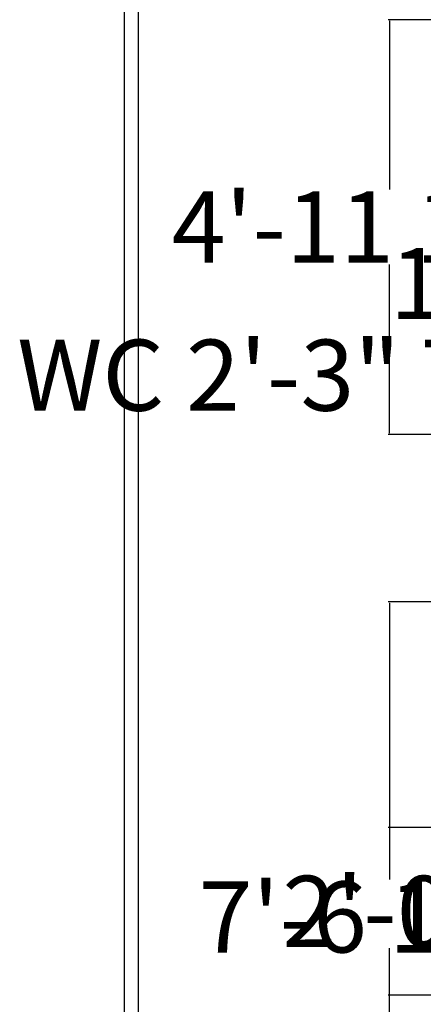
# Model space of a CAD drawing. Units: inches. Extents: x 1812 to 2791, y 2306 to 2959.
# Tile 3 of 8: x 1812 to 1870, y 2715 to 2856. Entities that reach past the tile are written whole.
import ezdxf

# ---------------------------------------------------------------- set-up
doc = ezdxf.new("R2010")
doc.units = ezdxf.units.IN
doc.layers.get('Defpoints').update_dxf_attribs({"lineweight": 50})
doc.layers.add('A-ANNO-DIMS', color=2, linetype='Continuous', lineweight=18)
doc.layers.add('A-ANNO-TTLB', color=7, linetype='Continuous', lineweight=25)
doc.styles.get("Standard").update_dxf_attribs({"font": 'arial.ttf'})
doc.dimstyles.get("Standard").update_dxf_attribs({"dimtxt": 10.18, "dimasz": 0.18, "dimexe": 0.18, "dimexo": 0.0625, "dimgap": 0.09, "dimtad": 0, "dimtih": 1, "dimtoh": 1, "dimdec": 0, "dimzin": 0, "dimdsep": 46, "dimlunit": 3, "dimtxsty": 'Standard', "dimcen": 0.09, "dimadec": 0, "dimazin": 0, "dimtfac": 1, "dimtdec": 0, "dimtofl": 0, "dimtmove": 0, "dimatfit": 3, "dimfxl": 1, "dimtolj": 1, "dimtzin": 0, "dimarcsym": 0})

# ---------------------------------------------------------------- blocks, each defined once
blk = doc.blocks.new('SHEET-FRAME-RESIDENCE')
blk.add_lwpolyline([(0.000131823559741, 632.8005012919775), (378.7609620870107, 632.8005012919775), (378.7609620870107, 0.0003856501880364), (0.000131823559741, 0.0003856501880364)], close=True)
blk.add_lwpolyline([(2.00013182355974, 71.32450104412055), (2.00013182355974, 630.8005012919775), (376.7609620870107, 630.8005012919775), (376.7609620870107, 71.32450104412055)])
blk = doc.blocks.new('*D56')
at = {"layer": 'A-ANNO-DIMS', "color": 0, "lineweight": -2, "transparency": 16777216}
for p, q in [((1900.14391049299, 2809.435242697527), (1900.14391049299, 2805.242430197514)), ((1927.312660493082, 2809.435242697527), (1927.312660493082, 2805.242430197514)), ((1900.14391049299, 2805.422430197514), (1899.96391049299, 2805.422430197514)), ((1927.132660493082, 2805.422430197514), (1900.323910492991, 2805.422430197514))]:
    blk.add_line(p, q, dxfattribs=at)
at = {"layer": 'A-ANNO-DIMS', "color": 0, "transparency": 16777216}
for points in [[(1900.323910492991, 2805.452430197514), (1900.323910492991, 2805.392430197514), (1900.14391049299, 2805.422430197514)], [(1927.132660493082, 2805.452430197514), (1927.132660493082, 2805.392430197514), (1927.312660493082, 2805.422430197514)]]:
    blk.add_solid(points, dxfattribs=at)
at = {"layer": 'Defpoints', "color": 0, "transparency": 16777216}
for p in [(1900.14391049299, 2809.497742697527), (1927.312660493082, 2809.497742697527), (1900.14391049299, 2805.422430197514)]:
    blk.add_point(p, dxfattribs=at)
at = {"layer": 'A-ANNO-DIMS', "color": 0, "transparency": 16777216, "insert": (1854.817341598038, 2805.422430197514), "char_height": 10.18, "attachment_point": 5}
blk.add_mtext('\\A1;WC 2\'-3" TYP.', dxfattribs=at)
blk = doc.blocks.new('*D57')
at = {"layer": 'A-ANNO-DIMS', "color": 0, "lineweight": -2, "transparency": 16777216}
for p, q in [((1900.081410492991, 2827.610242697545), (1895.888597992978, 2827.610242697545)), ((1896.068597992978, 2827.430242697545), (1896.068597992978, 2823.841625712543)), ((1896.068597992978, 2809.677742697528), (1896.068597992978, 2813.266359682529)), ((1900.081410492991, 2809.497742697528), (1895.888597992978, 2809.497742697528))]:
    blk.add_line(p, q, dxfattribs=at)
at = {"layer": 'A-ANNO-DIMS', "color": 0, "transparency": 16777216}
for points in [[(1896.038597992978, 2827.430242697545), (1896.098597992978, 2827.430242697545), (1896.068597992978, 2827.610242697545)], [(1896.038597992978, 2809.677742697528), (1896.098597992978, 2809.677742697528), (1896.068597992978, 2809.497742697528)]]:
    blk.add_solid(points, dxfattribs=at)
at = {"layer": 'Defpoints', "color": 0, "transparency": 16777216}
for p in [(1896.068597992978, 2827.610242697545), (1900.143910492991, 2827.610242697545), (1900.143910492991, 2809.497742697528)]:
    blk.add_point(p, dxfattribs=at)
at = {"layer": 'A-ANNO-DIMS', "color": 0, "transparency": 16777216, "insert": (1896.068597992979, 2818.553992697535), "char_height": 10.18, "attachment_point": 5}
blk.add_mtext('\\A1;1\'-6" TYP.', dxfattribs=at)
blk = doc.blocks.new('*D77')
at = {"layer": 'A-ANNO-DIMS', "color": 0, "lineweight": -2, "transparency": 16777216}
for p, q in [((1890.364364000001, 2856.361730000001), (1864.780736000002, 2856.361730000001)), ((1864.960736000002, 2856.181730000001), (1864.960736000002, 2832.008068137109)), ((1864.960736000002, 2797.127203000001), (1864.960736000002, 2821.300864862894)), ((1890.395003000001, 2796.947203000001), (1864.780736000002, 2796.947203000001))]:
    blk.add_line(p, q, dxfattribs=at)
at = {"layer": 'A-ANNO-DIMS', "color": 0, "transparency": 16777216}
for points in [[(1864.930736000002, 2856.181730000001), (1864.990736000002, 2856.181730000001), (1864.960736000002, 2856.361730000001)], [(1864.930736000002, 2797.127203000001), (1864.990736000002, 2797.127203000001), (1864.960736000002, 2796.947203000001)]]:
    blk.add_solid(points, dxfattribs=at)
at = {"layer": 'Defpoints', "color": 0, "transparency": 16777216}
for p in [(1890.426864000001, 2856.361730000001), (1864.960736000002, 2796.947203000001), (1890.457503000001, 2796.947203000001)]:
    blk.add_point(p, dxfattribs=at)
at = {"layer": 'A-ANNO-DIMS', "color": 0, "transparency": 16777216, "insert": (1864.960736000002, 2826.6544665), "char_height": 10.18, "attachment_point": 5}
blk.add_mtext('\\A1;4\'-11 1/2"', dxfattribs=at)
blk = doc.blocks.new('*D78')
at = {"layer": 'A-ANNO-DIMS', "color": 0, "lineweight": -2, "transparency": 16777216}
for p, q in [((1890.395003000001, 2772.947203000001), (1864.780736000002, 2772.947203000001)), ((1864.960736000002, 2772.767203000001), (1864.960736000002, 2733.146461637109)), ((1864.960736000002, 2682.818517000001), (1864.960736000002, 2722.439258362893)), ((1890.148236000001, 2682.638517000001), (1864.780736000002, 2682.638517000001))]:
    blk.add_line(p, q, dxfattribs=at)
at = {"layer": 'A-ANNO-DIMS', "color": 0, "transparency": 16777216}
for points in [[(1864.930736000002, 2772.767203000001), (1864.990736000002, 2772.767203000001), (1864.960736000002, 2772.947203000001)], [(1864.930736000002, 2682.818517000001), (1864.990736000002, 2682.818517000001), (1864.960736000002, 2682.638517000001)]]:
    blk.add_solid(points, dxfattribs=at)
at = {"layer": 'Defpoints', "color": 0, "transparency": 16777216}
for p in [(1890.457503000001, 2772.947203000001), (1864.960736000002, 2682.638517000001), (1890.210736000001, 2682.638517000001)]:
    blk.add_point(p, dxfattribs=at)
at = {"layer": 'A-ANNO-DIMS', "color": 0, "transparency": 16777216, "insert": (1864.960736000002, 2727.79286), "char_height": 10.18, "attachment_point": 5}
blk.add_mtext('\\A1;7\'-6 1/2"', dxfattribs=at)
blk = doc.blocks.new('*D81')
at = {"layer": 'A-ANNO-DIMS', "color": 0, "lineweight": -2, "transparency": 16777216}
for p, q in [((2011.324042000001, 2740.602944000001), (1864.780736000002, 2740.602944000001)), ((1864.960736000002, 2740.422944000001), (1864.960736000002, 2733.890577015008)), ((1864.960736000002, 2716.782944000001), (1864.960736000002, 2723.315310984994)), ((2011.324042000001, 2716.602944000002), (1864.780736000002, 2716.602944000002))]:
    blk.add_line(p, q, dxfattribs=at)
at = {"layer": 'A-ANNO-DIMS', "color": 0, "transparency": 16777216}
for points in [[(1864.930736000002, 2740.422944000001), (1864.990736000002, 2740.422944000001), (1864.960736000002, 2740.602944000001)], [(1864.930736000002, 2716.782944000001), (1864.990736000002, 2716.782944000001), (1864.960736000002, 2716.602944000002)]]:
    blk.add_solid(points, dxfattribs=at)
at = {"layer": 'Defpoints', "color": 0, "transparency": 16777216}
for p in [(2011.386542000001, 2740.602944000001), (1864.960736000002, 2716.602944000002), (2011.386542000001, 2716.602944000002)]:
    blk.add_point(p, dxfattribs=at)
at = {"layer": 'A-ANNO-DIMS', "color": 0, "transparency": 16777216, "insert": (1864.960736000002, 2728.602944), "char_height": 10.18, "attachment_point": 5}
blk.add_mtext('\\A1;2\'-0"', dxfattribs=at)

msp = doc.modelspace()

# ---------------------------------------------------------------- block references
at = {"layer": 'A-ANNO-TTLB'}
msp.add_blockref('SHEET-FRAME-RESIDENCE', (1827.027, 2306.124), dxfattribs=at)

# ---------------------------------------------------------------- dimensions: what is measured, and where the dimension line sits
at = {"layer": 'A-ANNO-DIMS'}
for base, p1, p2, picture, middle in [((1864.960736000002, 2796.947203000001), (1890.426864, 2856.36173), (1890.457503, 2796.947203), '*D77', (1864.960736000002, 2826.6544665)), ((1864.960736000002, 2682.638517000001), (1890.457503, 2772.947203000001), (1890.210736, 2682.638517), '*D78', (1864.960736000002, 2727.79286)), ((1864.960736000002, 2716.602944000002), (2011.386542, 2740.602944), (2011.386542, 2716.602944), '*D81', (1864.960736000002, 2728.602944))]:
    dim = msp.add_linear_dim(base=base, p1=p1, p2=p2, angle=90, dimstyle='Standard', override={"dimdec": 1, "dimlfac": 1, "dimrnd": 0, "dimzin": 1, "dimdsep": 46, "dimlunit": 4, "dimfrac": 2}, dxfattribs=at)
    dim.commit()
    dim.dimension.update_dxf_attribs({"geometry": picture, "text_midpoint": middle})
for base, p1, p2, angle, text, picture, middle in [((1896.068597992978, 2827.610242697545), (1900.14391049299, 2809.497742697527), (1900.14391049299, 2827.610242697544), 90, '<> TYP.', '*D57', (1896.068597992979, 2818.553992697535)), ((1900.14391049299, 2805.422430197514), (1927.312660493082, 2809.497742697527), (1900.14391049299, 2809.497742697527), 180, 'WC <> TYP.', '*D56', (1854.817341598038, 2805.422430197514))]:
    dim = msp.add_linear_dim(base=base, p1=p1, p2=p2, angle=angle, text=text, dimstyle='Standard', override={"dimdec": 1, "dimlfac": 1, "dimrnd": 0, "dimzin": 1, "dimdsep": 46, "dimlunit": 4, "dimfrac": 2}, dxfattribs=at)
    dim.commit()
    dim.dimension.update_dxf_attribs({"geometry": picture, "text_midpoint": middle})

doc.saveas('drawing.dxf')
